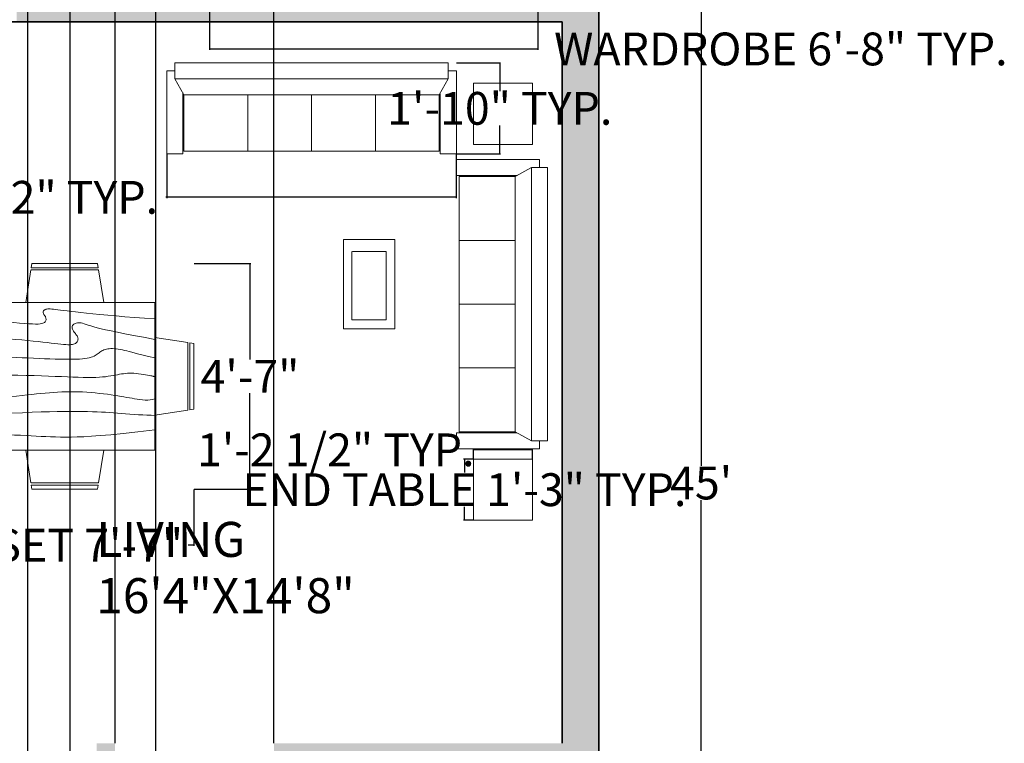
# Model space of a CAD drawing. Units: inches. Extents: x -4737294 to -4736756, y 1716389 to 1717040.
# Tile 22 of 25: x -4736996 to -4736756, y 1716669 to 1716845. Entities that reach past the tile are written whole.
import ezdxf

# ---------------------------------------------------------------- set-up
doc = ezdxf.new("R2010")
doc.units = ezdxf.units.IN
doc.header["$MEASUREMENT"] = 0
for name, color, linetype, lineweight in [('A-ANNO-DIMS', 2, 'Continuous', 18), ('A-AREA-IDEN', 250, 'Continuous', 18), ('A-WALL-PATT', 244, 'Continuous', 13), ('doors', 252, 'Continuous', 25), ('furniture', 250, 'Continuous', 18), ('walls', 252, 'Continuous', 35)]:
    doc.layers.add(name, color=color, linetype=linetype, lineweight=lineweight)
doc.styles.get("Standard").update_dxf_attribs({"font": 'arial.ttf'})
doc.dimstyles.get("Standard").update_dxf_attribs({"dimtxt": 8, "dimasz": 0.18, "dimexe": 0.18, "dimexo": 0.0625, "dimgap": 0.09, "dimtad": 0, "dimtih": 1, "dimtoh": 1, "dimzin": 0, "dimdsep": 46, "dimlunit": 3, "dimtxsty": 'Standard', "dimcen": 0.09, "dimadec": 0, "dimazin": 0, "dimtfac": 1, "dimtofl": 0, "dimtmove": 0, "dimatfit": 3, "dimfxl": 1, "dimtolj": 1, "dimtzin": 0, "dimarcsym": 0})

# ---------------------------------------------------------------- blocks, each defined once
blk = doc.blocks.new('*D22')
at = {"layer": 'A-ANNO-DIMS', "color": 0, "lineweight": -2, "transparency": 16777216}
for p, q in [((-4736855.08, 1717002.06), (-4736830.06, 1717002.06)), ((-4736830.24, 1717001.88), (-4736830.24, 1716736.22)), ((-4736830.24, 1716462.24), (-4736830.24, 1716727.91)), ((-4736855.08, 1716462.06), (-4736830.06, 1716462.06))]:
    blk.add_line(p, q, dxfattribs=at)
at = {"layer": 'A-ANNO-DIMS', "color": 0, "transparency": 16777216}
for points in [[(-4736830.27, 1717001.88), (-4736830.21, 1717001.88), (-4736830.24, 1717002.06)], [(-4736830.27, 1716462.24), (-4736830.21, 1716462.24), (-4736830.24, 1716462.06)]]:
    blk.add_solid(points, dxfattribs=at)
at = {"layer": 'Defpoints', "color": 0, "transparency": 16777216}
for p in [(-4736855.14, 1717002.06), (-4736830.24, 1717002.06), (-4736855.14, 1716462.06)]:
    blk.add_point(p, dxfattribs=at)
at = {"layer": 'A-ANNO-DIMS', "color": 0, "transparency": 16777216, "insert": (-4736830.24, 1716732.06), "char_height": 8, "attachment_point": 5}
blk.add_mtext("\\A1;45'", dxfattribs=at)
blk = doc.blocks.new('Dining Set - 36 x 72 in.')
for p, q in [((-22, 27.5), (-22.1562, 26.50042)), ((-5.8416, 26.5), (-22.1534, 26.5)), ((-22, 27.5), (-6, 27.5)), ((-5.8437, 26.49966), (-6, 27.5)), ((6, 27.5), (5.8438, 26.50042)), ((22.1584, 26.5), (5.8466, 26.5)), ((6, 27.5), (22, 27.5)), ((22.1563, 26.49966), (22, 27.5)), ((-22.2343, 26.00059), (-23.4847, 17.99762)), ((-22.2304, 26), (-5.7608, 26)), ((-4.5152, 17.99762), (-5.7655, 25.99926)), ((5.7657, 26.00059), (4.5153, 17.99762)), ((5.7696, 26), (22.2392, 26)), ((23.4848, 17.99762), (22.2345, 25.99926)), ((36, 18), (-36, 18)), ((-36, 18), (-36, -18)), ((36, -18), (36, 18)), ((-45.5, 8), (-44.5004, 8.15617)), ((-45.5, 8), (-45.5, -8)), ((-44.5, -8.15843), (-44.5, 8.15338)), ((-44.0006, 8.23428), (-35.9976, 9.48474)), ((-44, 8.23041), (-44, -8.23915)), ((44.0006, 8.23428), (35.9976, 9.48474)), ((44, 8.23041), (44, -8.23915)), ((44.5, -8.15843), (44.5, 8.15338)), ((45.5, 8), (44.5005, 8.15617)), ((45.5, 8), (45.5, -8)), ((-44.4997, -8.15631), (-45.5, -8)), ((-35.9976, -9.48476), (-43.9993, -8.2345)), ((35.9976, -9.48476), (43.9993, -8.2345)), ((44.4997, -8.15631), (45.5, -8)), ((-36, -18), (36, -18)), ((-22.2343, -26.0006), (-23.4847, -17.99762)), ((-4.5152, -17.99762), (-5.7655, -25.99928)), ((5.7657, -26.0006), (4.5153, -17.99762)), ((23.4848, -17.99762), (22.2345, -25.99928)), ((-22.2304, -26), (-5.7608, -26)), ((5.7696, -26), (22.2392, -26)), ((-22, -27.5), (-22.1562, -26.50044)), ((-5.8416, -26.5), (-22.1534, -26.5)), ((-22, -27.5), (-6, -27.5)), ((-5.8437, -26.49967), (-6, -27.5)), ((6, -27.5), (5.8438, -26.50044)), ((22.1584, -26.5), (5.8466, -26.5)), ((6, -27.5), (22, -27.5)), ((22.1563, -26.49967), (22, -27.5))]:
    blk.add_line(p, q)
for points in [[(-36, 15), (-31.1772, 14.97754), (-26.8079, 14.91406), (-22.8538, 14.81543), (-19.276, 14.6875), (-16.0362, 14.53613), (-13.0957, 14.36718), (-10.4159, 14.18652), (-7.9583, 14), (-5.6904, 13.81315), (-3.6035, 13.63021), (-1.6954, 13.45508), (0.0365, 13.29166), (1.5945, 13.14388), (2.9811, 13.01562), (4.1988, 12.9108), (5.25, 12.83333), (6.1393, 12.78613), (6.8802, 12.76823), (7.4883, 12.77767), (7.9792, 12.8125), (8.3685, 12.87077), (8.6719, 12.95052), (8.9049, 13.0498), (9.0833, 13.16666), (9.2205, 13.29899), (9.3216, 13.44401), (9.3895, 13.59879), (9.4271, 13.76041), (9.4373, 13.92594), (9.4232, 14.09245), (9.3875, 14.257), (9.3333, 14.41666), (9.2638, 14.56917), (9.1836, 14.71484), (9.0975, 14.85465), (9.0104, 14.98958), (8.9272, 15.1206), (8.8529, 15.2487), (8.7922, 15.37483), (8.75, 15.5), (8.7305, 15.62467), (8.7344, 15.74739), (8.7617, 15.86621), (8.8125, 15.97916), (8.8867, 16.08431), (8.9844, 16.17968), (9.1055, 16.26334), (9.25, 16.33333), (9.4189, 16.38802), (9.6172, 16.42708), (9.8506, 16.45052), (10.125, 16.45833), (10.4463, 16.45052), (10.8203, 16.42708), (11.2529, 16.38802), (11.75, 16.33333), (12.3184, 16.26318), (12.9694, 16.17838), (13.7151, 16.07991), (14.5677, 15.96875), (15.5395, 15.84586), (16.6426, 15.71224), (17.8893, 15.56884), (19.2917, 15.41666), (20.859, 15.25667), (22.5879, 15.08984), (24.4721, 14.91715), (26.5052, 14.73958), (28.6809, 14.5581), (30.9929, 14.3737), (33.4347, 14.18733), (36, 14)], [(-36, 10), (-28.9766, 10.14274), (-23.1725, 10.20442), (-18.4241, 10.19775), (-14.5677, 10.13541), (-11.4399, 10.03011), (-8.877, 9.89453), (-6.7154, 9.74137), (-4.7917, 9.58333), (-2.9698, 9.43082), (-1.2246, 9.28515), (0.4415, 9.14534), (2.026, 9.01041), (3.5266, 8.87939), (4.9408, 8.7513), (6.266, 8.62516), (7.5, 8.5), (8.6411, 8.37549), (9.6914, 8.2539), (10.6538, 8.13818), (11.5312, 8.03125), (12.3267, 7.93603), (13.043, 7.85547), (13.6831, 7.79248), (14.25, 7.75), (14.7471, 7.7303), (15.1797, 7.73307), (15.5537, 7.75732), (15.875, 7.80208), (16.1494, 7.86637), (16.3828, 7.94922), (16.5811, 8.04964), (16.75, 8.16666), (16.8944, 8.29915), (17.0143, 8.44531), (17.1089, 8.60319), (17.1771, 8.77083), (17.218, 8.94629), (17.2305, 9.1276), (17.2137, 9.31282), (17.1667, 9.5), (17.0895, 9.6875), (16.987, 9.875), (16.8649, 10.0625), (16.7292, 10.25), (16.5856, 10.4375), (16.4401, 10.625), (16.2985, 10.8125), (16.1667, 11), (16.05, 11.18733), (15.9518, 11.3737), (15.8752, 11.5581), (15.8229, 11.73958), (15.798, 11.91715), (15.8034, 12.08984), (15.842, 12.25667), (15.9167, 12.41666), (16.0295, 12.56836), (16.1784, 12.70833), (16.3605, 12.83268), (16.5729, 12.9375), (16.8127, 13.01888), (17.0768, 13.07291), (17.3625, 13.0957), (17.6667, 13.08333), (17.9894, 13.03312), (18.3418, 12.94726), (18.7382, 12.82918), (19.1927, 12.68229), (19.7195, 12.51001), (20.3327, 12.31575), (21.0465, 12.10294), (21.875, 11.875), (22.8357, 11.63354), (23.959, 11.37304), (25.2786, 11.08618), (26.8282, 10.76562), (28.6414, 10.40405), (30.752, 9.99414), (33.1936, 9.52856), (36, 9)], [(-36, 5.5), (-30.7157, 5.3348), (-26.069, 5.20963), (-21.9946, 5.11767), (-18.4271, 5.05208), (-15.3009, 5.00602), (-12.5508, 4.97265), (-10.1112, 4.94515), (-7.9167, 4.91666), (-5.909, 4.88167), (-4.0586, 4.83984), (-2.3429, 4.79215), (-0.7396, 4.73958), (0.7739, 4.6831), (2.22, 4.6237), (3.6213, 4.56233), (5, 4.5), (6.373, 4.43782), (7.7344, 4.3776), (9.0723, 4.32129), (10.375, 4.27083), (11.6309, 4.22819), (12.8281, 4.19531), (13.9551, 4.17415), (15, 4.16666), (15.954, 4.17448), (16.819, 4.19791), (17.6001, 4.23698), (18.3021, 4.29166), (18.9299, 4.36198), (19.4883, 4.44791), (19.9823, 4.54948), (20.4167, 4.66666), (20.7969, 4.79899), (21.1302, 4.94401), (21.4245, 5.09879), (21.6875, 5.26041), (21.9271, 5.42594), (22.1511, 5.59245), (22.3672, 5.757), (22.5834, 5.91666), (22.8065, 6.06868), (23.0404, 6.21093), (23.2879, 6.34147), (23.5521, 6.45833), (23.8358, 6.55957), (24.142, 6.64323), (24.4735, 6.70735), (24.8334, 6.75), (25.2235, 6.76969), (25.642, 6.76692), (26.0858, 6.74267), (26.5521, 6.69791), (27.0379, 6.63362), (27.5404, 6.55078), (28.0565, 6.45036), (28.5834, 6.33333), (29.1242, 6.19987), (29.7071, 6.04687), (30.3661, 5.87044), (31.1354, 5.66666), (32.0493, 5.43164), (33.142, 5.16146), (34.4475, 4.85221), (36, 4.5)], [(-36, -1), (-30.7915, -0.6591), (-26.0195, -0.38216), (-21.6519, -0.16284), (-17.6563, 0.00521), (-14.0005, 0.12833), (-10.6523, 0.21289), (-7.5796, 0.26522), (-4.75, 0.29166), (-2.134, 0.29793), (0.2878, 0.28711), (2.5317, 0.26163), (4.6146, 0.22396), (6.5529, 0.17651), (8.3633, 0.12174), (10.0623, 0.06209), (11.6667, 0), (13.1899, -0.06201), (14.6341, -0.1211), (15.9982, -0.17432), (17.2813, -0.21875), (18.4823, -0.25147), (19.6003, -0.26953), (20.6343, -0.27002), (21.5834, -0.25), (22.4481, -0.20768), (23.2357, -0.14584), (23.9549, -0.06836), (24.6146, 0.02083), (25.2235, 0.11784), (25.7904, 0.21875), (26.3241, 0.31966), (26.8334, 0.41666), (27.3265, 0.50618), (27.8099, 0.58593), (28.2894, 0.65397), (28.7709, 0.70833), (29.2601, 0.74707), (29.763, 0.76823), (30.2855, 0.76985), (30.8334, 0.75), (31.4088, 0.70784), (31.9994, 0.64713), (32.589, 0.57275), (33.1615, 0.48958), (33.7008, 0.4025), (34.1908, 0.3164), (34.6153, 0.23616), (34.9584, 0.16666), (35.2099, 0.11165), (35.3848, 0.07031), (35.504, 0.04069), (35.5886, 0.02083), (35.6594, 0.00879), (35.7377, 0.0026), (35.8442, 0.00032), (36, 0)], [(-36, -6.5), (-27.1843, -6.31267), (-20.084, -6.1263), (-14.469, -5.9419), (-10.1094, -5.76042), (-6.7752, -5.58285), (-4.2363, -5.41016), (-2.2629, -5.24333), (-0.625, -5.08334), (0.8708, -4.93099), (2.2715, -4.78646), (3.5872, -4.64974), (4.8281, -4.52084), (6.0046, -4.39974), (7.127, -4.28646), (8.2053, -4.18099), (9.25, -4.08334), (10.2705, -3.99382), (11.2734, -3.91407), (12.2647, -3.84603), (13.25, -3.79167), (14.2354, -3.75293), (15.2266, -3.73177), (16.2295, -3.73015), (17.25, -3.75), (18.2912, -3.79248), (19.3451, -3.85547), (20.4009, -3.93604), (21.4479, -4.03125), (22.4754, -4.13819), (23.4727, -4.25391), (24.4289, -4.37549), (25.3334, -4.5), (26.1785, -4.62492), (26.9694, -4.74935), (27.7145, -4.87281), (28.4219, -4.99479), (29.1, -5.11483), (29.7572, -5.23242), (30.4016, -5.34709), (31.0417, -5.45834), (31.6837, -5.56437), (32.3262, -5.65821), (32.9658, -5.73153), (33.599, -5.77604), (34.2224, -5.78345), (34.8327, -5.74545), (35.4264, -5.65373), (36, -5.5)], [(-36, -10), (-26.4022, -9.81299), (-18.4675, -9.62891), (-11.9839, -9.45069), (-6.7396, -9.28125), (-2.5226, -9.12354), (0.8789, -8.98047), (3.6769, -8.85498), (6.0833, -8.75), (8.2767, -8.66765), (10.3021, -8.60677), (12.1712, -8.56543), (13.8958, -8.54167), (15.4876, -8.53353), (16.9583, -8.53907), (18.3197, -8.55632), (19.5834, -8.58334), (20.7616, -8.61841), (21.8685, -8.66081), (22.9188, -8.71004), (23.9271, -8.76563), (24.9081, -8.82707), (25.8763, -8.89388), (26.8465, -8.96558), (27.8334, -9.04167), (28.8474, -9.12118), (29.8828, -9.20117), (30.93, -9.27824), (31.9792, -9.34896), (33.0205, -9.40991), (34.0443, -9.45768), (35.0407, -9.48885), (36, -9.5)], [(-36, -14.5), (-30.0881, -14.33513), (-25.0332, -14.21224), (-20.7312, -14.12647), (-17.0781, -14.07292), (-13.97, -14.04671), (-11.3027, -14.04297), (-8.9724, -14.05681), (-6.875, -14.08334), (-4.9224, -14.11833), (-3.0905, -14.16016), (-1.3709, -14.20785), (0.2448, -14.26042), (1.7647, -14.3169), (3.1973, -14.3763), (4.5507, -14.43767), (5.8333, -14.5), (7.0554, -14.5621), (8.235, -14.62175), (9.3922, -14.67652), (10.5469, -14.72396), (11.7192, -14.76164), (12.929, -14.78711), (14.1965, -14.79794), (15.5417, -14.79167), (16.9933, -14.76424), (18.6152, -14.70508), (20.4804, -14.60197), (22.6615, -14.44271), (25.2312, -14.21509), (28.2624, -13.9069), (31.8277, -13.50594), (36, -13)]]:
    blk.add_lwpolyline(points)
blk = doc.blocks.new('FABRIC SOFA 4S')
at = {"layer": 'furniture'}
for p, q in [((3, 54), (34, 54)), ((3, 51), (3, 54)), ((34, 48), (34, 54)), ((0, -51), (0, 51)), ((6, 51), (0, 51)), ((6, -51), (6, 51)), ((12, 47.63), (6, 51)), ((11.14, 48), (34, 48)), ((33, 23.81), (12, 23.81)), ((33, 0), (12, 0)), ((33, -23.81), (12, -23.81)), ((6, -51), (12, -47.63)), ((6, -51), (0, -51)), ((3, -54), (3, -51)), ((11.54, -48), (34, -48)), ((34, -48), (34, -54)), ((3, -54), (34, -54))]:
    blk.add_line(p, q, dxfattribs=at)
blk.add_lwpolyline([(12, -47.63), (12, 47.63), (33, 47.63), (33, -47.63)], close=True, dxfattribs=at)
blk = doc.blocks.new('*U20')
for p, q in [((0, 0), (0, -6)), ((40, 0), (40, -6))]:
    blk.add_line(p, q)
blk.add_lwpolyline([(0, 0), (0, 40), (1.75, 40), (1.75, 0)], close=True)
blk.add_arc((0, 0), 40, 0, 90)
blk = doc.blocks.new('TABLE-SOFA-END')
for p, q in [((0, 0), (0, 14.95)), ((0, 14.95), (14.41, 14.95)), ((14.41, 14.95), (14.41, 0)), ((0, 0), (14.41, 0))]:
    blk.add_line(p, q)
blk = doc.blocks.new('*D45')
at = {"layer": 'A-ANNO-DIMS', "color": 0, "lineweight": -2, "transparency": 16777216}
for p, q in [((-4736960.53, 1716812.27), (-4736960.53, 1716801.56)), ((-4736889.92, 1716812.27), (-4736889.92, 1716801.56)), ((-4736960.53, 1716801.74), (-4736960.71, 1716801.74)), ((-4736890.1, 1716801.74), (-4736960.35, 1716801.74))]:
    blk.add_line(p, q, dxfattribs=at)
at = {"layer": 'A-ANNO-DIMS', "color": 0, "transparency": 16777216}
for points in [[(-4736960.35, 1716801.77), (-4736960.35, 1716801.71), (-4736960.53, 1716801.74)], [(-4736890.1, 1716801.77), (-4736890.1, 1716801.71), (-4736889.92, 1716801.74)]]:
    blk.add_solid(points, dxfattribs=at)
at = {"layer": 'Defpoints', "color": 0, "transparency": 16777216}
for p in [(-4736960.53, 1716812.33), (-4736889.92, 1716812.33), (-4736960.53, 1716801.74)]:
    blk.add_point(p, dxfattribs=at)
at = {"layer": 'A-ANNO-DIMS', "color": 0, "transparency": 16777216, "insert": (-4737014.36, 1716801.74), "char_height": 8, "attachment_point": 5}
blk.add_mtext('\\A1;SOFA 5\'-10 1/2" TYP.', dxfattribs=at)
blk = doc.blocks.new('*D46')
at = {"layer": 'A-ANNO-DIMS', "color": 0, "lineweight": -2, "transparency": 16777216}
for p, q in [((-4736889.86, 1716834.56), (-4736879.15, 1716834.56)), ((-4736879.33, 1716834.38), (-4736879.33, 1716827.62)), ((-4736879.33, 1716812.51), (-4736879.33, 1716819.27)), ((-4736889.86, 1716812.33), (-4736879.15, 1716812.33))]:
    blk.add_line(p, q, dxfattribs=at)
at = {"layer": 'A-ANNO-DIMS', "color": 0, "transparency": 16777216}
for points in [[(-4736879.36, 1716834.38), (-4736879.3, 1716834.38), (-4736879.33, 1716834.56)], [(-4736879.36, 1716812.51), (-4736879.3, 1716812.51), (-4736879.33, 1716812.33)]]:
    blk.add_solid(points, dxfattribs=at)
at = {"layer": 'Defpoints', "color": 0, "transparency": 16777216}
for p in [(-4736889.92, 1716834.56), (-4736889.92, 1716812.33), (-4736879.33, 1716812.33)]:
    blk.add_point(p, dxfattribs=at)
at = {"layer": 'A-ANNO-DIMS', "color": 0, "transparency": 16777216, "insert": (-4736879.33, 1716823.44), "char_height": 8, "attachment_point": 5}
blk.add_mtext('\\A1;1\'-10" TYP.', dxfattribs=at)
blk = doc.blocks.new('*D47')
at = {"layer": 'A-ANNO-DIMS', "color": 0, "lineweight": -2, "transparency": 16777216}
for p, q in [((-4736950.1, 1716849.87), (-4736950.1, 1716837.75)), ((-4736870.07, 1716849.87), (-4736870.07, 1716837.75)), ((-4736949.92, 1716837.93), (-4736870.25, 1716837.93)), ((-4736870.07, 1716837.93), (-4736869.89, 1716837.93))]:
    blk.add_line(p, q, dxfattribs=at)
at = {"layer": 'A-ANNO-DIMS', "color": 0, "transparency": 16777216}
for points in [[(-4736949.92, 1716837.96), (-4736949.92, 1716837.9), (-4736950.1, 1716837.93)], [(-4736870.25, 1716837.96), (-4736870.25, 1716837.9), (-4736870.07, 1716837.93)]]:
    blk.add_solid(points, dxfattribs=at)
at = {"layer": 'Defpoints', "color": 0, "transparency": 16777216}
for p in [(-4736950.1, 1716849.93), (-4736870.07, 1716849.93), (-4736870.07, 1716837.93)]:
    blk.add_point(p, dxfattribs=at)
at = {"layer": 'A-ANNO-DIMS', "color": 0, "transparency": 16777216, "insert": (-4736810.8, 1716837.93), "char_height": 8, "attachment_point": 5}
blk.add_mtext('\\A1;WARDROBE 6\'-8" TYP.', dxfattribs=at)
blk = doc.blocks.new('*D51')
at = {"layer": 'A-ANNO-DIMS', "color": 0, "lineweight": -2, "transparency": 16777216}
for p, q in [((-4736885.78, 1716737.91), (-4736888.14, 1716737.91)), ((-4736887.96, 1716737.73), (-4736887.96, 1716734.61)), ((-4736887.96, 1716723.14), (-4736887.96, 1716726.26)), ((-4736885.78, 1716722.96), (-4736888.14, 1716722.96))]:
    blk.add_line(p, q, dxfattribs=at)
at = {"layer": 'A-ANNO-DIMS', "color": 0, "transparency": 16777216}
for points in [[(-4736887.99, 1716737.73), (-4736887.93, 1716737.73), (-4736887.96, 1716737.91)], [(-4736887.99, 1716723.14), (-4736887.93, 1716723.14), (-4736887.96, 1716722.96)]]:
    blk.add_solid(points, dxfattribs=at)
at = {"layer": 'Defpoints', "color": 0, "transparency": 16777216}
for p in [(-4736885.72, 1716737.91), (-4736887.96, 1716722.96), (-4736885.72, 1716722.96)]:
    blk.add_point(p, dxfattribs=at)
at = {"layer": 'A-ANNO-DIMS', "color": 0, "transparency": 16777216, "insert": (-4736887.96, 1716730.43), "char_height": 8, "attachment_point": 5}
blk.add_mtext('\\A1;END TABLE 1\'-3" TYP.', dxfattribs=at)
blk = doc.blocks.new('*D52')
at = {"layer": 'A-ANNO-DIMS', "color": 0, "lineweight": -2, "transparency": 16777216}
for p, q in [((-4736885.72, 1716740.15), (-4736885.9, 1716740.15)), ((-4736885.72, 1716737.97), (-4736885.72, 1716740.33)), ((-4736871.49, 1716740.15), (-4736885.54, 1716740.15)), ((-4736871.31, 1716737.97), (-4736871.31, 1716740.33))]:
    blk.add_line(p, q, dxfattribs=at)
at = {"layer": 'A-ANNO-DIMS', "color": 0, "transparency": 16777216}
for points in [[(-4736885.54, 1716740.18), (-4736885.54, 1716740.12), (-4736885.72, 1716740.15)], [(-4736871.49, 1716740.18), (-4736871.49, 1716740.12), (-4736871.31, 1716740.15)]]:
    blk.add_solid(points, dxfattribs=at)
at = {"layer": 'Defpoints', "color": 0, "transparency": 16777216}
for p in [(-4736885.72, 1716740.15), (-4736885.72, 1716737.91), (-4736871.31, 1716737.91)]:
    blk.add_point(p, dxfattribs=at)
at = {"layer": 'A-ANNO-DIMS', "color": 0, "transparency": 16777216, "insert": (-4736919.32, 1716740.15), "char_height": 8, "attachment_point": 5}
blk.add_mtext('\\A1;1\'-2 1/2" TYP.', dxfattribs=at)
blk = doc.blocks.new('*D53')
at = {"layer": 'A-ANNO-DIMS', "color": 0, "lineweight": -2, "transparency": 16777216}
for p, q in [((-4737044.89, 1716730.5), (-4737044.89, 1716716.73)), ((-4736953.89, 1716730.5), (-4736953.89, 1716716.73)), ((-4737044.71, 1716716.91), (-4737043.44, 1716716.91)), ((-4736954.07, 1716716.91), (-4736955.34, 1716716.91))]:
    blk.add_line(p, q, dxfattribs=at)
at = {"layer": 'A-ANNO-DIMS', "color": 0, "transparency": 16777216}
for points in [[(-4737044.71, 1716716.94), (-4737044.71, 1716716.88), (-4737044.89, 1716716.91)], [(-4736954.07, 1716716.94), (-4736954.07, 1716716.88), (-4736953.89, 1716716.91)]]:
    blk.add_solid(points, dxfattribs=at)
at = {"layer": 'Defpoints', "color": 0, "transparency": 16777216}
for p in [(-4737044.89, 1716730.56), (-4736953.89, 1716730.56), (-4736953.89, 1716716.91)]:
    blk.add_point(p, dxfattribs=at)
at = {"layer": 'A-ANNO-DIMS', "color": 0, "transparency": 16777216, "insert": (-4736999.39, 1716716.91), "char_height": 8, "attachment_point": 5}
blk.add_mtext('\\A1;DINING SET 7\'-7"', dxfattribs=at)
blk = doc.blocks.new('*D54')
at = {"layer": 'A-ANNO-DIMS', "color": 0, "lineweight": -2, "transparency": 16777216}
for p, q in [((-4736953.83, 1716785.56), (-4736940.06, 1716785.56)), ((-4736940.24, 1716785.38), (-4736940.24, 1716762.15)), ((-4736940.24, 1716730.74), (-4736940.24, 1716753.97)), ((-4736953.83, 1716730.56), (-4736940.06, 1716730.56))]:
    blk.add_line(p, q, dxfattribs=at)
at = {"layer": 'A-ANNO-DIMS', "color": 0, "transparency": 16777216}
for points in [[(-4736940.27, 1716785.38), (-4736940.21, 1716785.38), (-4736940.24, 1716785.56)], [(-4736940.27, 1716730.74), (-4736940.21, 1716730.74), (-4736940.24, 1716730.56)]]:
    blk.add_solid(points, dxfattribs=at)
at = {"layer": 'Defpoints', "color": 0, "transparency": 16777216}
for p in [(-4736953.89, 1716785.56), (-4736940.24, 1716785.56), (-4736953.89, 1716730.56)]:
    blk.add_point(p, dxfattribs=at)
at = {"layer": 'A-ANNO-DIMS', "color": 0, "transparency": 16777216, "insert": (-4736940.24, 1716758.06), "char_height": 8, "attachment_point": 5}
blk.add_mtext('\\A1;4\'-7"', dxfattribs=at)
blk = doc.blocks.new('*D64')
at = {"layer": 'A-ANNO-DIMS', "color": 0, "lineweight": -2, "transparency": 16777216}
for p, q in [((-4736994.45, 1716844.5), (-4736994.45, 1716423.69)), ((-4736963.28, 1716844.5), (-4736963.28, 1716423.69)), ((-4736994.27, 1716423.87), (-4736989.65, 1716423.87)), ((-4736963.46, 1716423.87), (-4736968.07, 1716423.87))]:
    blk.add_line(p, q, dxfattribs=at)
at = {"layer": 'A-ANNO-DIMS', "color": 0, "transparency": 16777216}
for points in [[(-4736994.27, 1716423.9), (-4736994.27, 1716423.84), (-4736994.45, 1716423.87)], [(-4736963.46, 1716423.9), (-4736963.46, 1716423.84), (-4736963.28, 1716423.87)]]:
    blk.add_solid(points, dxfattribs=at)
at = {"layer": 'Defpoints', "color": 0, "transparency": 16777216}
for p in [(-4736994.45, 1716844.56), (-4736963.28, 1716844.56), (-4736963.28, 1716423.87)]:
    blk.add_point(p, dxfattribs=at)
at = {"layer": 'A-ANNO-DIMS', "color": 0, "transparency": 16777216, "insert": (-4736978.86, 1716423.87), "char_height": 8, "attachment_point": 5}
blk.add_mtext('\\A1;2\'-7"', dxfattribs=at)
blk = doc.blocks.new('*D65')
at = {"layer": 'A-ANNO-DIMS', "color": 0, "lineweight": -2, "transparency": 16777216}
for p, q in [((-4737007.1, 1716596.13), (-4737007.1, 1717035.24)), ((-4737006.92, 1717035.06), (-4736984.27, 1717035.06)), ((-4736984.09, 1716596.13), (-4736984.09, 1717035.24)), ((-4736984.09, 1717035.06), (-4736983.91, 1717035.06))]:
    blk.add_line(p, q, dxfattribs=at)
at = {"layer": 'A-ANNO-DIMS', "color": 0, "transparency": 16777216}
for points in [[(-4737006.92, 1717035.09), (-4737006.92, 1717035.03), (-4737007.1, 1717035.06)], [(-4736984.27, 1717035.09), (-4736984.27, 1717035.03), (-4736984.09, 1717035.06)]]:
    blk.add_solid(points, dxfattribs=at)
at = {"layer": 'Defpoints', "color": 0, "transparency": 16777216}
for p in [(-4736984.09, 1717035.06), (-4737007.1, 1716596.06), (-4736984.09, 1716596.06)]:
    blk.add_point(p, dxfattribs=at)
at = {"layer": 'A-ANNO-DIMS', "color": 0, "transparency": 16777216, "insert": (-4736970.46, 1717035.06), "char_height": 8, "attachment_point": 5}
blk.add_mtext('\\A1;1\'-11"', dxfattribs=at)
blk = doc.blocks.new('*D66')
at = {"layer": 'A-ANNO-DIMS', "color": 0, "lineweight": -2, "transparency": 16777216}
for p, q in [((-4736973.14, 1716668.63), (-4736973.14, 1717035.24)), ((-4736972.96, 1717035.06), (-4736964.49, 1717035.06)), ((-4736934.57, 1717035.06), (-4736943.05, 1717035.06)), ((-4736934.39, 1716668.63), (-4736934.39, 1717035.24))]:
    blk.add_line(p, q, dxfattribs=at)
at = {"layer": 'A-ANNO-DIMS', "color": 0, "transparency": 16777216}
for points in [[(-4736972.96, 1717035.09), (-4736972.96, 1717035.03), (-4736973.14, 1717035.06)], [(-4736934.57, 1717035.09), (-4736934.57, 1717035.03), (-4736934.39, 1717035.06)]]:
    blk.add_solid(points, dxfattribs=at)
at = {"layer": 'Defpoints', "color": 0, "transparency": 16777216}
for p in [(-4736934.39, 1717035.06), (-4736973.14, 1716668.56), (-4736934.39, 1716668.56)]:
    blk.add_point(p, dxfattribs=at)
at = {"layer": 'A-ANNO-DIMS', "color": 0, "transparency": 16777216, "insert": (-4736953.77, 1717035.06), "char_height": 8, "attachment_point": 5}
blk.add_mtext('\\A1;3\'-3"', dxfattribs=at)

msp = doc.modelspace()

# ---------------------------------------------------------------- hatches: boundary and pattern name
at = {"layer": 'A-WALL-PATT'}
h = msp.add_hatch(color=256, dxfattribs=at)
h.dxf.hatch_style = 1
h.paths.add_polyline_path([(-4737206.144, 1716844.565), (-4737110.144, 1716844.565), (-4737110.144, 1716823.907), (-4737105.644, 1716823.907), (-4737105.644, 1716844.565), (-4737098.44, 1716844.565), (-4737098.44, 1716849.065), (-4737206.144, 1716849.065), (-4737206.144, 1716993.065), (-4736864.144, 1716993.065), (-4736864.144, 1716849.065), (-4736963.275, 1716849.065), (-4736994.446, 1716849.065), (-4736997.144, 1716849.065), (-4736997.144, 1716844.565), (-4736864.144, 1716844.565), (-4736864.144, 1716668.565), (-4736934.391, 1716668.565), (-4736934.391, 1716664.065), (-4736864.144, 1716664.065), (-4736864.144, 1716462.065), (-4736855.144, 1716462.065), (-4736855.144, 1717002.065), (-4737215.144, 1717002.065), (-4737215.144, 1716462.065), (-4737206.144, 1716462.065), (-4737206.144, 1716659.065), (-4737062.144, 1716659.065), (-4737062.144, 1716647.493), (-4737057.644, 1716647.493), (-4737057.644, 1716796.565), (-4737071.812, 1716796.565), (-4737071.812, 1716792.065), (-4737070.805, 1716792.065), (-4737062.144, 1716792.065), (-4737062.144, 1716668.065), (-4737206.144, 1716668.065), (-4737206.144, 1716792.065), (-4737093.784, 1716792.065), (-4737093.784, 1716796.565), (-4737206.144, 1716796.565)])
h = msp.add_hatch(color=256, dxfattribs=at)
h.dxf.hatch_style = 1
h.paths.add_polyline_path([(-4737057.644, 1716600.884), (-4737062.144, 1716600.884), (-4737062.144, 1716534.565), (-4736933.144, 1716534.565), (-4736933.144, 1716462.065), (-4736924.144, 1716462.065), (-4736924.144, 1716543.565), (-4736973.144, 1716543.565), (-4736973.144, 1716668.565), (-4736977.644, 1716668.565), (-4736977.644, 1716543.565), (-4737057.644, 1716543.565), (-4737057.644, 1716591.565), (-4737007.073, 1716591.565), (-4737007.073, 1716596.065), (-4737057.644, 1716596.065)])
h.paths.add_polyline_path([(-4736962.872, 1716471.065), (-4737062.144, 1716471.065), (-4737062.144, 1716462.065), (-4736962.872, 1716462.065)], flags=17)
h.paths.add_polyline_path([(-4737161.883, 1716716.26), (-4737096.689, 1716716.26), (-4737096.689, 1716729.349), (-4737161.883, 1716729.349)], flags=9)
h.paths.add_polyline_path([(-4737161.912, 1716729.958), (-4737095.809, 1716729.958), (-4737095.809, 1716743.222), (-4737161.912, 1716743.222)], flags=9)
h.paths.add_polyline_path([(-4736943.842, 1716913.818), (-4736878.647, 1716913.818), (-4736878.647, 1716926.907), (-4736943.842, 1716926.907)], flags=9)
h.paths.add_polyline_path([(-4736943.871, 1716927.516), (-4736877.767, 1716927.516), (-4736877.767, 1716940.78), (-4736943.871, 1716940.78)], flags=9)
h = msp.add_hatch(color=256, dxfattribs=at)
h.dxf.hatch_style = 1
h.paths.add_polyline_path([(-4736994.446, 1716849.065), (-4736997.144, 1716849.065), (-4736997.144, 1716844.565), (-4736994.446, 1716844.565)])
h.paths.add_polyline_path([(-4737023.821, 1716917.161), (-4737023.821, 1716880.778), (-4737014.648, 1716880.778), (-4737014.648, 1716917.161)], flags=9)
h.paths.add_polyline_path([(-4737014.221, 1716917.181), (-4737014.221, 1716884.798), (-4737004.926, 1716884.798), (-4737004.926, 1716917.181)], flags=9)

# ---------------------------------------------------------------- linework, layer by layer
at = {"layer": 'furniture'}
for p, q in [((-4736917.415, 1716769.648), (-4736917.415, 1716791.464)), ((-4736917.415, 1716791.464), (-4736904.902, 1716791.464)), ((-4736917.415, 1716791.464), (-4736917.415, 1716769.648)), ((-4736904.902, 1716791.464), (-4736917.415, 1716791.464)), ((-4736904.902, 1716791.464), (-4736904.902, 1716769.648)), ((-4736904.902, 1716769.648), (-4736904.902, 1716791.464)), ((-4736915.424, 1716771.818), (-4736915.424, 1716788.523)), ((-4736915.222, 1716788.523), (-4736907.063, 1716788.523)), ((-4736907.063, 1716788.523), (-4736907.063, 1716771.818)), ((-4736907.063, 1716771.818), (-4736915.424, 1716771.818)), ((-4736904.902, 1716769.648), (-4736917.415, 1716769.648)), ((-4736917.415, 1716769.648), (-4736904.902, 1716769.648))]:
    msp.add_line(p, q, dxfattribs=at)
at = {"layer": 'walls'}
for p, q in [((-4736855.144, 1717002.065), (-4736855.144, 1716462.065)), ((-4737105.644, 1716844.565), (-4736864.144, 1716844.565)), ((-4736864.144, 1716844.565), (-4736864.144, 1716668.565))]:
    msp.add_line(p, q, dxfattribs=at)

# ---------------------------------------------------------------- block references
at = {"layer": 'doors', "xscale": 0.7792671805443983, "yscale": 0.7792671805443983, "zscale": 0.7792671805443983}
msp.add_blockref('*U20', (-4736994.446, 1716849.24), dxfattribs=at)
at = {"layer": 'furniture', "xscale": -0.6537939928824033, "yscale": 0.6537939928824033, "zscale": 0.6537939928824033}
for p, rotation in [((-4736925.223, 1716834.558), 89.9999999998931), ((-4736867.689, 1716775.676), 359.9999999998932)]:
    msp.add_blockref('FABRIC SOFA 4S', p, dxfattribs=dict(at, rotation=rotation))
at = {"layer": 'furniture'}
for name, p in [('TABLE-SOFA-END', (-4736885.72, 1716814.617)), ('Dining Set - 36 x 72 in.', (-4736999.39, 1716758.063))]:
    msp.add_blockref(name, p, dxfattribs=at)
at = {"layer": 'furniture', "rotation": 180}
msp.add_blockref('TABLE-SOFA-END', (-4736871.309, 1716737.906), dxfattribs=at)

# ---------------------------------------------------------------- texts
at = {"layer": 'A-AREA-IDEN'}
for s, height, p in [('LIVING', 8.5453, (-4736977.704, 1716714.035)), ('16\'4"X14\'8"', 8.54529, (-4736977.704, 1716700.307))]:
    msp.add_text(s, height=height, dxfattribs=at).set_placement(p)

# ---------------------------------------------------------------- dimensions: what is measured, and where the dimension line sits
at = {"layer": 'A-ANNO-DIMS'}
for base, p1, p2, picture, middle in [((-4736984.094, 1717035.065), (-4737007.097, 1716596.065), (-4736984.094, 1716596.065), '*D65', (-4736970.46, 1717035.065)), ((-4736934.391, 1717035.065), (-4736973.144, 1716668.565), (-4736934.391, 1716668.565), '*D66', (-4736953.768, 1717035.065)), ((-4736963.275, 1716423.869), (-4736994.446, 1716844.565), (-4736963.275, 1716844.565), '*D64', (-4736978.861, 1716423.869))]:
    dim = msp.add_linear_dim(base=base, p1=p1, p2=p2, dimstyle='Standard', override={"dimdec": 1, "dimlfac": 1, "dimrnd": 0, "dimzin": 1, "dimdsep": 46, "dimlunit": 4, "dimfrac": 2}, dxfattribs=at)
    dim.commit()
    dim.dimension.update_dxf_attribs({"geometry": picture, "text_midpoint": middle})
for base, p1, p2, override, picture, middle in [((-4736830.238, 1717002.065), (-4736855.144, 1716462.065), (-4736855.144, 1717002.065), {"dimclrd": 0, "dimclre": 0, "dimclrt": 0}, '*D22', (-4736830.238, 1716732.065)), ((-4736940.24, 1716785.563), (-4736953.89, 1716730.563), (-4736953.89, 1716785.563), {"dimdec": 1, "dimlfac": 1, "dimrnd": 0, "dimzin": 1, "dimdsep": 46, "dimlunit": 4, "dimfrac": 2}, '*D54', (-4736940.24, 1716758.063))]:
    dim = msp.add_linear_dim(base=base, p1=p1, p2=p2, angle=90, dimstyle='Standard', override=override, dxfattribs=at)
    dim.commit()
    dim.dimension.update_dxf_attribs({"geometry": picture, "text_midpoint": middle})
for base, p1, p2, text, picture, middle in [((-4736870.074, 1716837.93), (-4736950.098, 1716849.933), (-4736870.074, 1716849.933), 'WARDROBE <> TYP.', '*D47', (-4736810.797, 1716837.93)), ((-4736953.89, 1716716.913), (-4737044.89, 1716730.563), (-4736953.89, 1716730.563), 'DINING SET <>', '*D53', (-4736999.39, 1716716.913))]:
    dim = msp.add_linear_dim(base=base, p1=p1, p2=p2, text=text, dimstyle='Standard', override={"dimdec": 1, "dimlfac": 1, "dimrnd": 0, "dimzin": 1, "dimdsep": 46, "dimlunit": 4, "dimfrac": 2}, dxfattribs=at)
    dim.commit()
    dim.dimension.update_dxf_attribs({"geometry": picture, "text_midpoint": middle})
for base, p1, p2, angle, text, picture, middle in [((-4736879.327, 1716812.329), (-4736889.918, 1716834.558), (-4736889.918, 1716812.329), 270, '<> TYP.', '*D46', (-4736879.327, 1716823.444)), ((-4736960.528, 1716801.738), (-4736889.918, 1716812.329), (-4736960.528, 1716812.329), 180, 'SOFA <> TYP.', '*D45', (-4737014.356, 1716801.738)), ((-4736885.72, 1716740.148), (-4736871.309, 1716737.906), (-4736885.72, 1716737.906), 180, '<> TYP.', '*D52', (-4736919.316, 1716740.148)), ((-4736887.962, 1716722.96), (-4736885.72, 1716737.906), (-4736885.72, 1716722.96), 270, 'END TABLE <> TYP.', '*D51', (-4736887.962, 1716730.433))]:
    dim = msp.add_linear_dim(base=base, p1=p1, p2=p2, angle=angle, text=text, dimstyle='Standard', override={"dimdec": 1, "dimlfac": 1, "dimrnd": 0, "dimzin": 1, "dimdsep": 46, "dimlunit": 4, "dimfrac": 2}, dxfattribs=at)
    dim.commit()
    dim.dimension.update_dxf_attribs({"geometry": picture, "text_midpoint": middle})

doc.saveas('drawing.dxf')
